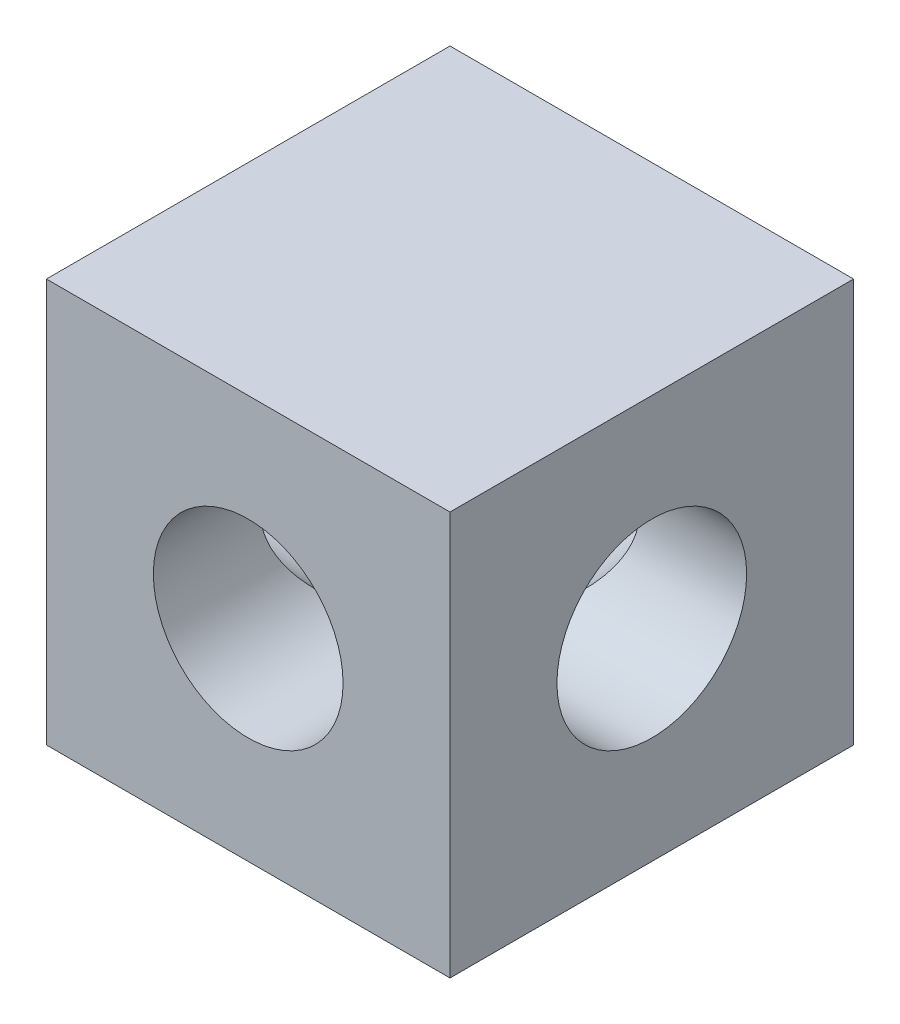
SolidWorks part; units mm, degrees
material "Plain Carbon Steel"
ref_plane "Front Plane" through (0, 0, 0) normal (0, 0, 1) x (1, 0, 0)
ref_plane "Top Plane" through (0, 0, 0) normal (0, 1, 0) x (1, 0, 0)
ref_plane "Right Plane" through (0, 0, 0) normal (1, 0, 0) x (0, 0, -1)
sketch "Block Profile 20.32 Square" plane through (0, 0, 0) normal (0, 1, 0) x (1, 0, 0)
  line L1 (-10.16, 10.16) -> (10.16, 10.16)
  line L2 (-10.16, 10.16) -> (-10.16, -10.16)
  line L3 (-10.16, -10.16) -> (10.16, -10.16)
  line L4 (10.16, 10.16) -> (10.16, -10.16)
  line L5 (-10.16, 10.16) -> (10.16, -10.16) construction
  line L6 (-10.16, -10.16) -> (10.16, 10.16) construction
  point P0 (0, 0)
  dimension "D1" = 20.32
  dimension "D2" = 20.32
extrude "Cube Block 20.32" add sketch "Block Profile 20.32 Square" along normal blind 20.32
sketch "Cross Hole A Profile" plane through (0, 0, 10.16) normal (0, 0, 1) x (1, 0, 0)
  line L0 (0, 20.32) -> (0, 0) construction
  line L1 (-10.16, 20.32) -> (10.16, 20.32) construction
  circle A0 centre (0, 10.16) radius 4.775
  dimension "D1" = 9.55
extrude "Cross Hole A Ø9.35" cut sketch "Cross Hole A Profile" against normal through all
sketch "Cross Hole B Profile" plane through (10.16, 0, 0) normal (1, 0, 0) x (0, 0, -1)
  line L0 (0, 0) -> (0, 20.32) construction
  line L1 (-10.16, 20.32) -> (10.16, 20.32) construction
  circle A0 centre (0, 10.16) radius 4.775
  dimension "D1" = 9.55
extrude "Cross Hole B Ø9.35" cut sketch "Cross Hole B Profile" against normal through all
